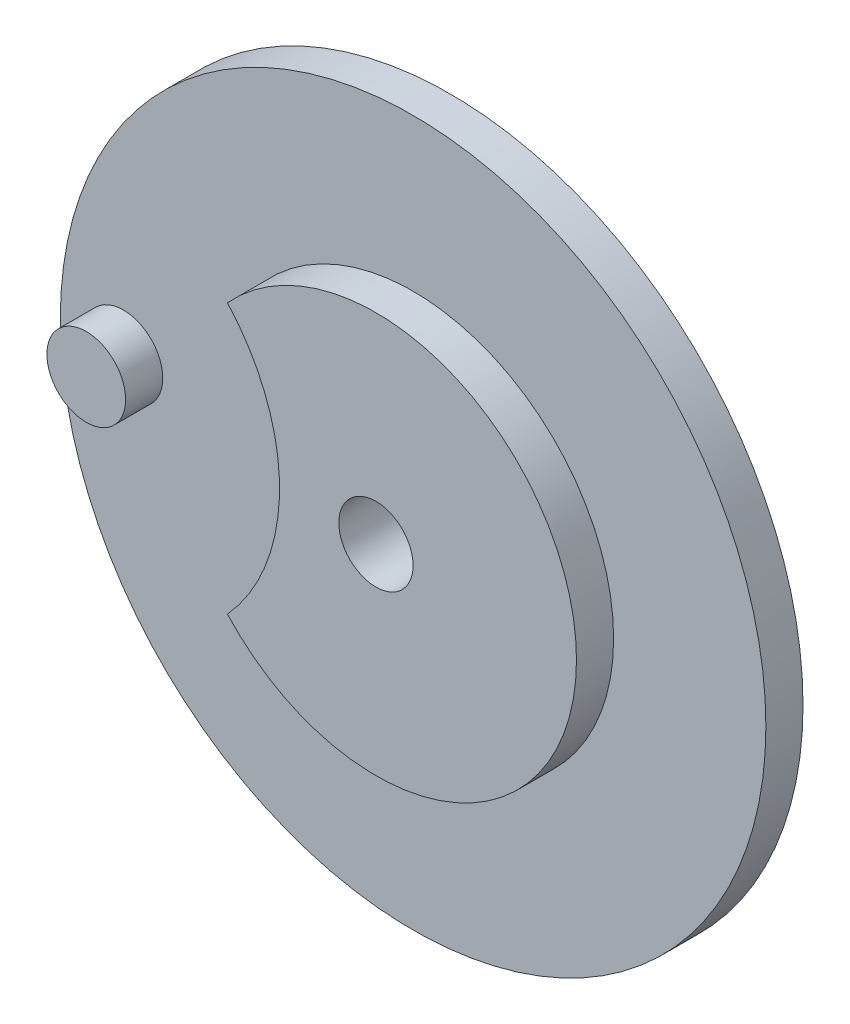
ISO-10303-21;
HEADER;
FILE_DESCRIPTION(('STEP AP214'),'2;1');
FILE_NAME('part.step','',(''),(''),'','','');
FILE_SCHEMA(('AUTOMOTIVE_DESIGN { 1 0 10303 214 1 1 1 1 }'));
ENDSEC;
DATA;
#1=APPLICATION_CONTEXT('core data for automotive mechanical design processes');
#2=APPLICATION_PROTOCOL_DEFINITION('international standard','automotive_design',2000,#1);
#3=PRODUCT_CONTEXT('',#1,'mechanical');
#4=PRODUCT('Part','Part','',(#3));
#5=PRODUCT_RELATED_PRODUCT_CATEGORY('part','',(#4));
#6=PRODUCT_DEFINITION_FORMATION('','',#4);
#7=PRODUCT_DEFINITION_CONTEXT('part definition',#1,'design');
#8=PRODUCT_DEFINITION('design','',#6,#7);
#9=PRODUCT_DEFINITION_SHAPE('','',#8);
#10=(LENGTH_UNIT() NAMED_UNIT(*) SI_UNIT(.MILLI.,.METRE.));
#11=(NAMED_UNIT(*) PLANE_ANGLE_UNIT() SI_UNIT($,.RADIAN.));
#12=(NAMED_UNIT(*) SI_UNIT($,.STERADIAN.) SOLID_ANGLE_UNIT());
#13=UNCERTAINTY_MEASURE_WITH_UNIT(LENGTH_MEASURE(1.E-05),#10,'distance_accuracy_value','');
#14=(GEOMETRIC_REPRESENTATION_CONTEXT(3) GLOBAL_UNCERTAINTY_ASSIGNED_CONTEXT((#13)) GLOBAL_UNIT_ASSIGNED_CONTEXT((#10,
#11,#12)) REPRESENTATION_CONTEXT('',''));
#15=CARTESIAN_POINT('',(0.,0.,0.));
#16=DIRECTION('',(0.,0.,1.));
#17=DIRECTION('',(1.,0.,0.));
#18=AXIS2_PLACEMENT_3D('',#15,#16,#17);
#19=CARTESIAN_POINT('',(0.,0.,-5.));
#20=DIRECTION('',(0.,0.,1.));
#21=DIRECTION('',(1.,0.,0.));
#22=AXIS2_PLACEMENT_3D('',#19,#20,#21);
#23=CYLINDRICAL_SURFACE('',#22,47.5);
#24=CARTESIAN_POINT('',(0.,0.,-5.));
#25=DIRECTION('',(0.,0.,1.));
#26=DIRECTION('',(1.,0.,0.));
#27=AXIS2_PLACEMENT_3D('',#24,#25,#26);
#28=CIRCLE('',#27,47.5);
#29=CARTESIAN_POINT('',(47.5,0.,-5.));
#30=VERTEX_POINT('',#29);
#31=EDGE_CURVE('E12',#30,#30,#28,.T.);
#32=ORIENTED_EDGE('',*,*,#31,.T.);
#33=EDGE_LOOP('',(#32));
#34=FACE_BOUND('',#33,.T.);
#35=CARTESIAN_POINT('',(0.,0.,0.));
#36=DIRECTION('',(0.,0.,1.));
#37=DIRECTION('',(1.,0.,0.));
#38=AXIS2_PLACEMENT_3D('',#35,#36,#37);
#39=CIRCLE('',#38,47.5);
#40=CARTESIAN_POINT('',(47.5,0.,0.));
#41=VERTEX_POINT('',#40);
#42=EDGE_CURVE('E49',#41,#41,#39,.T.);
#43=ORIENTED_EDGE('',*,*,#42,.F.);
#44=EDGE_LOOP('',(#43));
#45=FACE_BOUND('',#44,.T.);
#46=ADVANCED_FACE('F50',(#34,#45),#23,.T.);
#47=CARTESIAN_POINT('',(0.,0.,-5.));
#48=DIRECTION('',(0.,0.,1.));
#49=DIRECTION('',(1.,0.,0.));
#50=AXIS2_PLACEMENT_3D('',#47,#48,#49);
#51=PLANE('',#50);
#52=CARTESIAN_POINT('',(0.,0.,-5.));
#53=DIRECTION('',(0.,0.,1.));
#54=DIRECTION('',(1.,0.,0.));
#55=AXIS2_PLACEMENT_3D('',#52,#53,#54);
#56=CIRCLE('',#55,5.);
#57=CARTESIAN_POINT('',(5.,0.,-5.));
#58=VERTEX_POINT('',#57);
#59=EDGE_CURVE('E98',#58,#58,#56,.T.);
#60=ORIENTED_EDGE('',*,*,#59,.T.);
#61=EDGE_LOOP('',(#60));
#62=FACE_BOUND('',#61,.T.);
#63=ORIENTED_EDGE('',*,*,#31,.F.);
#64=EDGE_LOOP('',(#63));
#65=FACE_BOUND('',#64,.T.);
#66=ADVANCED_FACE('F106',(#62,#65),#51,.F.);
#67=CARTESIAN_POINT('',(0.,0.,0.));
#68=DIRECTION('',(0.,0.,1.));
#69=DIRECTION('',(1.,0.,0.));
#70=AXIS2_PLACEMENT_3D('',#67,#68,#69);
#71=PLANE('',#70);
#72=CARTESIAN_POINT('',(-39.,0.,0.));
#73=DIRECTION('',(0.,0.,1.));
#74=DIRECTION('',(1.,0.,0.));
#75=AXIS2_PLACEMENT_3D('',#72,#73,#74);
#76=CIRCLE('',#75,5.3);
#77=CARTESIAN_POINT('',(-33.7,0.,0.));
#78=VERTEX_POINT('',#77);
#79=EDGE_CURVE('E95',#78,#78,#76,.T.);
#80=ORIENTED_EDGE('',*,*,#79,.F.);
#81=EDGE_LOOP('',(#80));
#82=FACE_BOUND('',#81,.T.);
#83=CARTESIAN_POINT('',(-39.978464591939,0.,0.));
#84=DIRECTION('',(0.,0.,1.));
#85=DIRECTION('',(1.,0.,0.));
#86=AXIS2_PLACEMENT_3D('',#83,#84,#85);
#87=CIRCLE('',#86,27.);
#88=CARTESIAN_POINT('',(-19.9892322959695,-18.1502229247403,0.));
#89=VERTEX_POINT('',#88);
#90=CARTESIAN_POINT('',(-19.9892322959695,18.1502229247403,0.));
#91=VERTEX_POINT('',#90);
#92=EDGE_CURVE('E64',#89,#91,#87,.T.);
#93=ORIENTED_EDGE('',*,*,#92,.T.);
#94=CARTESIAN_POINT('',(0.,0.,0.));
#95=DIRECTION('',(0.,0.,1.));
#96=DIRECTION('',(1.,0.,0.));
#97=AXIS2_PLACEMENT_3D('',#94,#95,#96);
#98=CIRCLE('',#97,27.);
#99=EDGE_CURVE('E83',#89,#91,#98,.T.);
#100=ORIENTED_EDGE('',*,*,#99,.F.);
#101=EDGE_LOOP('',(#93,#100));
#102=FACE_BOUND('',#101,.T.);
#103=ORIENTED_EDGE('',*,*,#42,.T.);
#104=EDGE_LOOP('',(#103));
#105=FACE_BOUND('',#104,.T.);
#106=ADVANCED_FACE('F87',(#82,#102,#105),#71,.T.);
#107=CARTESIAN_POINT('',(0.,0.,-5.));
#108=DIRECTION('',(0.,0.,1.));
#109=DIRECTION('',(1.,0.,0.));
#110=AXIS2_PLACEMENT_3D('',#107,#108,#109);
#111=CYLINDRICAL_SURFACE('',#110,5.);
#112=ORIENTED_EDGE('',*,*,#59,.F.);
#113=EDGE_LOOP('',(#112));
#114=FACE_BOUND('',#113,.T.);
#115=CARTESIAN_POINT('',(0.,0.,5.));
#116=DIRECTION('',(0.,0.,1.));
#117=DIRECTION('',(1.,0.,0.));
#118=AXIS2_PLACEMENT_3D('',#115,#116,#117);
#119=CIRCLE('',#118,5.);
#120=CARTESIAN_POINT('',(5.,0.,5.));
#121=VERTEX_POINT('',#120);
#122=EDGE_CURVE('E77',#121,#121,#119,.T.);
#123=ORIENTED_EDGE('',*,*,#122,.T.);
#124=EDGE_LOOP('',(#123));
#125=FACE_BOUND('',#124,.T.);
#126=ADVANCED_FACE('F116',(#114,#125),#111,.F.);
#127=CARTESIAN_POINT('',(-39.978464591939,0.,5.));
#128=DIRECTION('',(0.,0.,-1.));
#129=DIRECTION('',(-1.,0.,0.));
#130=AXIS2_PLACEMENT_3D('',#127,#128,#129);
#131=CYLINDRICAL_SURFACE('',#130,27.);
#132=ORIENTED_EDGE('',*,*,#92,.F.);
#133=DIRECTION('',(0.,0.,-1.));
#134=VECTOR('',#133,1.);
#135=CARTESIAN_POINT('',(-19.9892322959695,-18.1502229247403,5.));
#136=LINE('',#135,#134);
#137=CARTESIAN_POINT('',(-19.9892322959695,-18.1502229247403,5.));
#138=VERTEX_POINT('',#137);
#139=EDGE_CURVE('E78',#138,#89,#136,.T.);
#140=ORIENTED_EDGE('',*,*,#139,.F.);
#141=CARTESIAN_POINT('',(-39.978464591939,0.,5.));
#142=DIRECTION('',(0.,0.,1.));
#143=DIRECTION('',(1.,0.,0.));
#144=AXIS2_PLACEMENT_3D('',#141,#142,#143);
#145=CIRCLE('',#144,27.);
#146=CARTESIAN_POINT('',(-19.9892322959695,18.1502229247403,5.));
#147=VERTEX_POINT('',#146);
#148=EDGE_CURVE('E76',#138,#147,#145,.T.);
#149=ORIENTED_EDGE('',*,*,#148,.T.);
#150=DIRECTION('',(0.,0.,-1.));
#151=VECTOR('',#150,1.);
#152=CARTESIAN_POINT('',(-19.9892322959695,18.1502229247403,5.));
#153=LINE('',#152,#151);
#154=EDGE_CURVE('E74',#147,#91,#153,.T.);
#155=ORIENTED_EDGE('',*,*,#154,.T.);
#156=EDGE_LOOP('',(#132,#140,#149,#155));
#157=FACE_BOUND('',#156,.T.);
#158=ADVANCED_FACE('F79',(#157),#131,.F.);
#159=CARTESIAN_POINT('',(0.,0.,5.));
#160=DIRECTION('',(0.,0.,-1.));
#161=DIRECTION('',(-1.,0.,0.));
#162=AXIS2_PLACEMENT_3D('',#159,#160,#161);
#163=CYLINDRICAL_SURFACE('',#162,27.);
#164=ORIENTED_EDGE('',*,*,#99,.T.);
#165=ORIENTED_EDGE('',*,*,#154,.F.);
#166=CARTESIAN_POINT('',(0.,0.,5.));
#167=DIRECTION('',(0.,0.,1.));
#168=DIRECTION('',(1.,0.,0.));
#169=AXIS2_PLACEMENT_3D('',#166,#167,#168);
#170=CIRCLE('',#169,27.);
#171=EDGE_CURVE('E69',#138,#147,#170,.T.);
#172=ORIENTED_EDGE('',*,*,#171,.F.);
#173=ORIENTED_EDGE('',*,*,#139,.T.);
#174=EDGE_LOOP('',(#164,#165,#172,#173));
#175=FACE_BOUND('',#174,.T.);
#176=ADVANCED_FACE('F84',(#175),#163,.T.);
#177=CARTESIAN_POINT('',(0.,0.,5.));
#178=DIRECTION('',(0.,0.,1.));
#179=DIRECTION('',(1.,0.,0.));
#180=AXIS2_PLACEMENT_3D('',#177,#178,#179);
#181=PLANE('',#180);
#182=ORIENTED_EDGE('',*,*,#148,.F.);
#183=ORIENTED_EDGE('',*,*,#171,.T.);
#184=EDGE_LOOP('',(#182,#183));
#185=FACE_BOUND('',#184,.T.);
#186=ORIENTED_EDGE('',*,*,#122,.F.);
#187=EDGE_LOOP('',(#186));
#188=FACE_BOUND('',#187,.T.);
#189=ADVANCED_FACE('F130',(#185,#188),#181,.T.);
#190=CARTESIAN_POINT('',(-39.,0.,5.));
#191=DIRECTION('',(0.,0.,-1.));
#192=DIRECTION('',(-1.,0.,0.));
#193=AXIS2_PLACEMENT_3D('',#190,#191,#192);
#194=CYLINDRICAL_SURFACE('',#193,5.3);
#195=CARTESIAN_POINT('',(-39.,0.,5.));
#196=DIRECTION('',(0.,0.,1.));
#197=DIRECTION('',(1.,0.,0.));
#198=AXIS2_PLACEMENT_3D('',#195,#196,#197);
#199=CIRCLE('',#198,5.3);
#200=CARTESIAN_POINT('',(-33.7,0.,5.));
#201=VERTEX_POINT('',#200);
#202=EDGE_CURVE('E90',#201,#201,#199,.T.);
#203=ORIENTED_EDGE('',*,*,#202,.F.);
#204=EDGE_LOOP('',(#203));
#205=FACE_BOUND('',#204,.T.);
#206=ORIENTED_EDGE('',*,*,#79,.T.);
#207=EDGE_LOOP('',(#206));
#208=FACE_BOUND('',#207,.T.);
#209=ADVANCED_FACE('F128',(#205,#208),#194,.T.);
#210=CARTESIAN_POINT('',(0.,0.,5.));
#211=DIRECTION('',(0.,0.,1.));
#212=DIRECTION('',(1.,0.,0.));
#213=AXIS2_PLACEMENT_3D('',#210,#211,#212);
#214=PLANE('',#213);
#215=ORIENTED_EDGE('',*,*,#202,.T.);
#216=EDGE_LOOP('',(#215));
#217=FACE_BOUND('',#216,.T.);
#218=ADVANCED_FACE('F135',(#217),#214,.T.);
#219=CLOSED_SHELL('',(#46,#66,#106,#126,#158,#176,#189,#209,#218));
#220=MANIFOLD_SOLID_BREP('B2',#219);
#221=ADVANCED_BREP_SHAPE_REPRESENTATION('',(#18,#220),#14);
#222=SHAPE_DEFINITION_REPRESENTATION(#9,#221);
ENDSEC;
END-ISO-10303-21;
